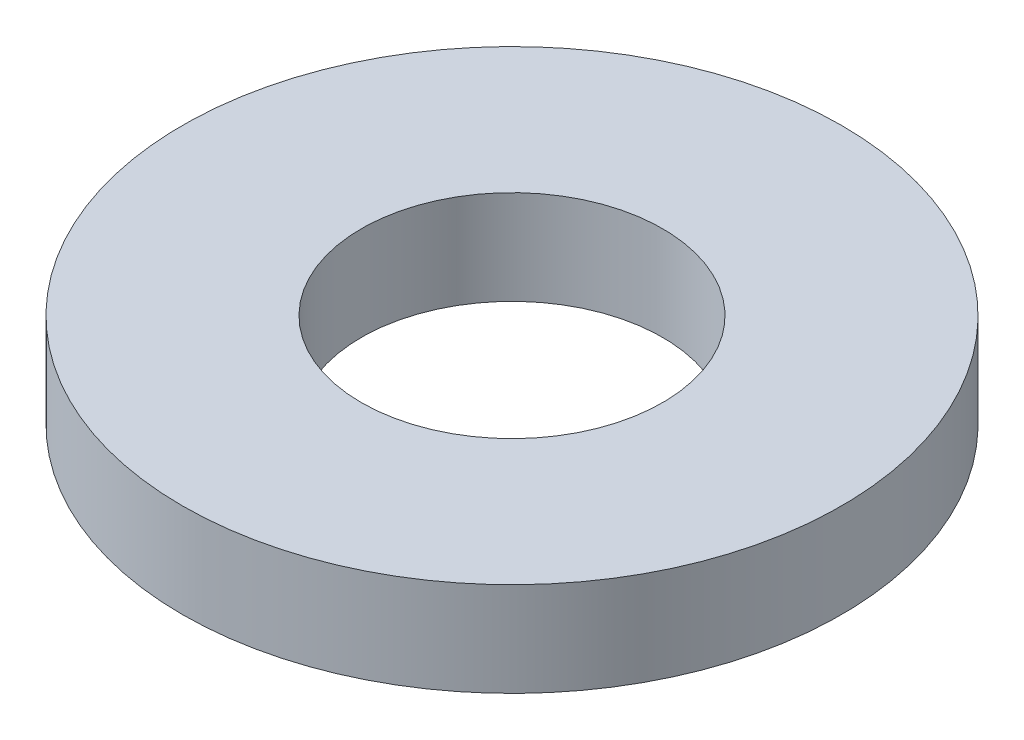
SolidWorks part; units mm, degrees
material "Plain Carbon Steel"
ref_plane "Front Plane" through (0, 0, 0) normal (0, 0, 1) x (1, 0, 0)
ref_plane "Top Plane" through (0, 0, 0) normal (0, 1, 0) x (1, 0, 0)
ref_plane "Right Plane" through (0, 0, 0) normal (1, 0, 0) x (0, 0, -1)
sketch "Washer Profile Ø35-Ø16" plane through (0, 0, 0) normal (0, 1, 0) x (1, 0, 0)
  circle A0 centre (0, 0) radius 8
  circle A1 centre (0, 0) radius 17.5
  dimension "D1" = 16
  dimension "D2" = 35
extrude "Washer Body 5mm" add sketch "Washer Profile Ø35-Ø16" along normal mid plane 5
